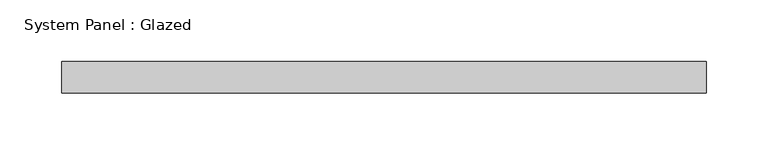
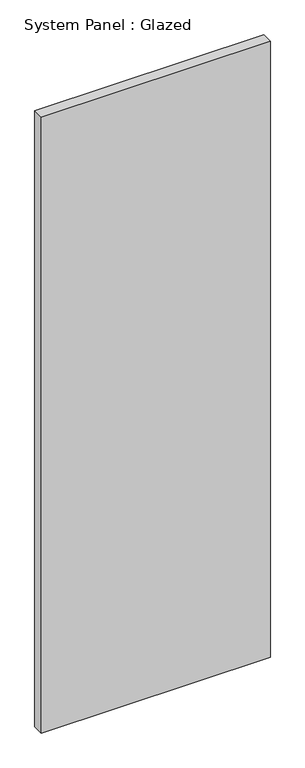
"""IFC4 building model written with IfcOpenShell, lengths in millimetres: plate geometry, System Panel : Glazed."""

from ifc_helpers import new_model, si_unit, origin, origin_with_axes, place, context, project, spatial, polyline, outline, extrude, source, transform, mapped, element, save


def system_panel_glazed_c23b727d(model_context):
    return source(origin(), model_context, "Body", "SweptSolid", [
        extrude(outline(polyline([(260.35, 19.05), (-260.35, 19.05), (-260.35, 44.45), (260.35, 44.45), (260.35, 19.05)])), origin_with_axes(), (0.0, 0.0, 1.0), 1479.2683749),
    ])


if __name__ == "__main__":
    model = new_model("IFC4")
    model_context = context("Model", 3, world=origin())
    ifc_project = project(units=[si_unit("LENGTHUNIT", "METRE", prefix="MILLI")], contexts=[model_context])
    site = spatial("IfcSite", under=ifc_project)
    building = spatial("IfcBuilding", under=site)
    placement = place(None, origin())
    system_panel_glazed_shape = system_panel_glazed_c23b727d(model_context)
    element("IfcPlate", 1, ObjectType="System Panel : Glazed", at=placement, inside=building, context=model_context, shape_type="MappedRepresentation", body=[
        mapped(system_panel_glazed_shape, transform((0.0, 0.0, 0.0), x_axis=(1.0, 0.0, 0.0), y_axis=(0.0, 1.0, 0.0), z_axis=(0.0, 0.0, 1.0))),
    ])
    save(model, "model.ifc")

# Revit data of these elements
# Type "System Panel : Glazed"
#   Construction Type Id = "GSP4R"
#   Analytic Construction = "1/8 in Pilkington single glazing"
#   Visual Light Transmittance = 0.9
#   Solar Heat Gain Coefficient = 0.86
#   Heat Transfer Coefficient (U) = 1.18115 BTU/(h·ft²·°F)
#   Define Thermal Properties by = 1
# Element 1 (IfcPlate, "System Panel : Glazed")
#   Materials on its faces: "Glass"
# Materials
#   "Glass": class "Glass", colour RGB 0 128 192, transparency 0.75, Description = "Soda Lime Glass", Cost = 0
